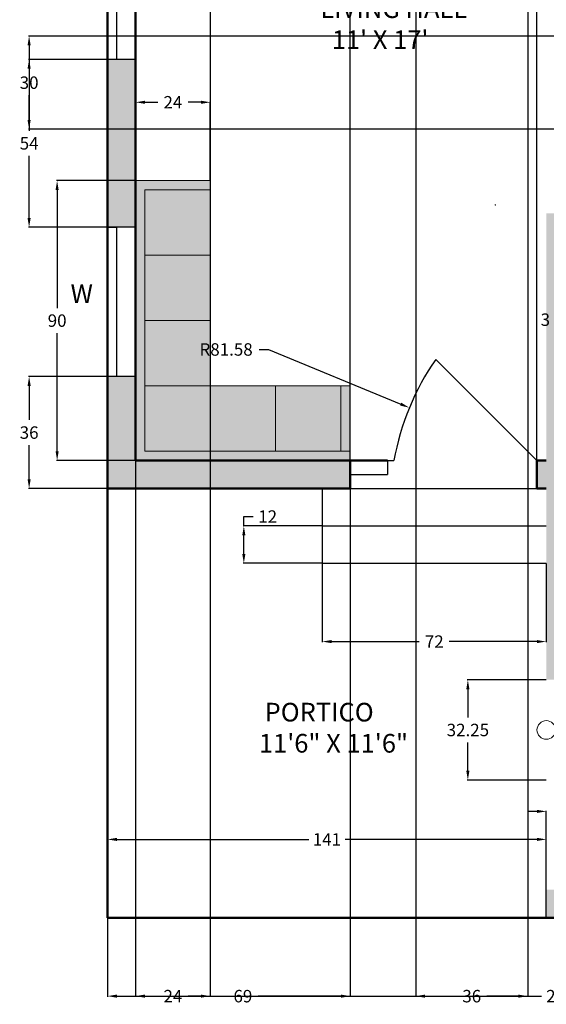
# Model space of a CAD drawing. Units: inches. Extents: x 30 to 385, y 81 to 626.
# Tile 1 of 4: x 30 to 199, y 81 to 398. Entities that reach past the tile are written whole.
import ezdxf

# ---------------------------------------------------------------- set-up
doc = ezdxf.new("R2010")
doc.units = ezdxf.units.IN
doc.header["$MEASUREMENT"] = 0
for name, color, linetype, lineweight in [('A-ANNO-DIMS', 2, 'Continuous', 18), ('A-ANNO-REF', 8, 'Continuous', 13), ('A-ANNO-SYMB', 7, 'Continuous', 18), ('A-ANNO-TEXT', 7, 'Continuous', 18), ('A-AREA-IDEN', 7, 'Continuous', 25), ('A-DOOR', 3, 'Continuous', 25), ('A-FLOR-STRS', 7, 'Continuous', 25), ('A-FURN', 8, 'Continuous', 18), ('A-GLAZ', 4, 'Continuous', 25), ('A-WALL', 7, 'Continuous', 50), ('A-WALL-PATT', 32, 'Continuous', 13)]:
    doc.layers.add(name, color=color, linetype=linetype, lineweight=lineweight)
doc.layers.add('A-FURN-PATT', color=254, linetype='Continuous', lineweight=13, true_color=0xfeeab9)
doc.styles.get("Standard").update_dxf_attribs({"font": 'arial.ttf'})
doc.dimstyles.get("Standard").update_dxf_attribs({"dimtxt": 4, "dimasz": 3, "dimexe": 0.18, "dimexo": 0.0625, "dimgap": 2, "dimtad": 0, "dimtih": 1, "dimtoh": 1, "dimdec": 0, "dimzin": 0, "dimdsep": 46, "dimlunit": 3, "dimtxsty": 'Standard', "dimcen": 0.09, "dimadec": 0, "dimazin": 0, "dimtfac": 1, "dimtdec": 0, "dimtofl": 0, "dimtmove": 0, "dimatfit": 3, "dimfxl": 1, "dimtolj": 1, "dimtzin": 0, "dimarcsym": 0})

# ---------------------------------------------------------------- blocks, each defined once
blk = doc.blocks.new('WIN-48')
for p, q in [((0, 0), (0, 9)), ((48, 0), (48, 9)), ((0, 6), (48, 6))]:
    blk.add_line(p, q)
blk = doc.blocks.new('*D16')
at = {"layer": 'A-ANNO-DIMS', "color": 0, "lineweight": -2, "transparency": 16777216}
for p, q in [((57.92, 109), (57.92, 83.68)), ((348.92, 109), (348.92, 83.68)), ((60.92, 83.86), (197.35, 83.86)), ((345.92, 83.86), (209.49, 83.86))]:
    blk.add_line(p, q, dxfattribs=at)
at = {"layer": 'A-ANNO-DIMS', "color": 0, "transparency": 16777216}
for points in [[(60.92, 84.36), (60.92, 83.36), (57.92, 83.86)], [(345.92, 84.36), (345.92, 83.36), (348.92, 83.86)]]:
    blk.add_solid(points, dxfattribs=at)
at = {"layer": 'Defpoints', "color": 0, "transparency": 16777216}
for p in [(57.92, 109.06), (348.92, 109.06), (348.92, 83.86)]:
    blk.add_point(p, dxfattribs=at)
at = {"layer": 'A-ANNO-DIMS', "color": 0, "transparency": 16777216, "insert": (203.42, 83.86), "char_height": 4, "attachment_point": 5}
blk.add_mtext('\\A1;291', dxfattribs=at)
blk = doc.blocks.new('*D18')
at = {"layer": 'A-ANNO-DIMS', "color": 0, "lineweight": -2, "transparency": 16777216}
for p, q in [((57.92, 109.13), (57.92, 134.44)), ((60.92, 134.26), (122.57, 134.26)), ((195.92, 134.26), (134.26, 134.26)), ((198.92, 109.13), (198.92, 134.44))]:
    blk.add_line(p, q, dxfattribs=at)
at = {"layer": 'A-ANNO-DIMS', "color": 0, "transparency": 16777216}
for points in [[(60.92, 134.76), (60.92, 133.76), (57.92, 134.26)], [(195.92, 134.76), (195.92, 133.76), (198.92, 134.26)]]:
    blk.add_solid(points, dxfattribs=at)
at = {"layer": 'Defpoints', "color": 0, "transparency": 16777216}
for p in [(198.92, 134.26), (57.92, 109.06), (198.92, 109.06)]:
    blk.add_point(p, dxfattribs=at)
at = {"layer": 'A-ANNO-DIMS', "color": 0, "transparency": 16777216, "insert": (128.42, 134.26), "char_height": 4, "attachment_point": 5}
blk.add_mtext('\\A1;141', dxfattribs=at)
blk = doc.blocks.new('*D23')
at = {"layer": 'A-ANNO-DIMS', "color": 0, "lineweight": -2, "transparency": 16777216}
for p, q in [((57.86, 283.06), (32.54, 283.06)), ((32.72, 280.06), (32.72, 269.11)), ((32.72, 250.06), (32.72, 261.02)), ((57.86, 247.06), (32.54, 247.06))]:
    blk.add_line(p, q, dxfattribs=at)
at = {"layer": 'A-ANNO-DIMS', "color": 0, "transparency": 16777216}
for points in [[(32.22, 280.06), (33.22, 280.06), (32.72, 283.06)], [(32.22, 250.06), (33.22, 250.06), (32.72, 247.06)]]:
    blk.add_solid(points, dxfattribs=at)
at = {"layer": 'Defpoints', "color": 0, "transparency": 16777216}
for p in [(32.72, 283.06), (57.92, 283.06), (57.92, 247.06)]:
    blk.add_point(p, dxfattribs=at)
at = {"layer": 'A-ANNO-DIMS', "color": 0, "transparency": 16777216, "insert": (32.72, 265.06), "char_height": 4, "attachment_point": 5}
blk.add_mtext('\\A1;36', dxfattribs=at)
blk = doc.blocks.new('*D24')
at = {"layer": 'A-ANNO-DIMS', "color": 0, "lineweight": -2, "transparency": 16777216}
for p, q in [((57.86, 385.06), (32.54, 385.06)), ((32.72, 382.06), (32.72, 362.1)), ((32.72, 334.06), (32.72, 354.03)), ((57.86, 331.06), (32.54, 331.06))]:
    blk.add_line(p, q, dxfattribs=at)
at = {"layer": 'A-ANNO-DIMS', "color": 0, "transparency": 16777216}
for points in [[(32.22, 382.06), (33.22, 382.06), (32.72, 385.06)], [(32.22, 334.06), (33.22, 334.06), (32.72, 331.06)]]:
    blk.add_solid(points, dxfattribs=at)
at = {"layer": 'Defpoints', "color": 0, "transparency": 16777216}
for p in [(32.72, 385.06), (57.92, 385.06), (57.92, 331.06)]:
    blk.add_point(p, dxfattribs=at)
at = {"layer": 'A-ANNO-DIMS', "color": 0, "transparency": 16777216, "insert": (32.72, 358.06), "char_height": 4, "attachment_point": 5}
blk.add_mtext('\\A1;54', dxfattribs=at)
blk = doc.blocks.new('*D28')
at = {"layer": 'A-ANNO-DIMS', "color": 0, "lineweight": -2, "transparency": 16777216}
for p, q in [((66.92, 469), (66.92, 83.68)), ((90.92, 469), (90.92, 83.68)), ((69.92, 83.86), (74.03, 83.86)), ((87.92, 83.86), (83.81, 83.86))]:
    blk.add_line(p, q, dxfattribs=at)
at = {"layer": 'A-ANNO-DIMS', "color": 0, "transparency": 16777216}
for points in [[(69.92, 84.36), (69.92, 83.36), (66.92, 83.86)], [(87.92, 84.36), (87.92, 83.36), (90.92, 83.86)]]:
    blk.add_solid(points, dxfattribs=at)
at = {"layer": 'Defpoints', "color": 0, "transparency": 16777216}
for p in [(66.92, 469.06), (90.92, 469.06), (90.92, 83.86)]:
    blk.add_point(p, dxfattribs=at)
at = {"layer": 'A-ANNO-DIMS', "color": 0, "transparency": 16777216, "insert": (78.92, 83.86), "char_height": 4, "attachment_point": 5}
blk.add_mtext('\\A1;24', dxfattribs=at)
blk = doc.blocks.new('*D32')
at = {"layer": 'A-ANNO-DIMS', "color": 0, "lineweight": -2, "transparency": 16777216}
for p, q in [((135.92, 247.13), (135.92, 623.44)), ((138.92, 623.26), (161.05, 623.26)), ((192.92, 623.26), (170.79, 623.26)), ((195.92, 247.13), (195.92, 623.44))]:
    blk.add_line(p, q, dxfattribs=at)
at = {"layer": 'A-ANNO-DIMS', "color": 0, "transparency": 16777216}
for points in [[(138.92, 623.76), (138.92, 622.76), (135.92, 623.26)], [(192.92, 623.76), (192.92, 622.76), (195.92, 623.26)]]:
    blk.add_solid(points, dxfattribs=at)
at = {"layer": 'Defpoints', "color": 0, "transparency": 16777216}
for p in [(195.92, 623.26), (135.92, 247.06), (195.92, 247.06)]:
    blk.add_point(p, dxfattribs=at)
at = {"layer": 'A-ANNO-DIMS', "color": 0, "transparency": 16777216, "insert": (165.92, 623.26), "char_height": 4, "attachment_point": 5}
blk.add_mtext('\\A1;60', dxfattribs=at)
blk = doc.blocks.new('*D33')
at = {"layer": 'A-ANNO-DIMS', "color": 0, "lineweight": -2, "transparency": 16777216}
for p, q in [((156.96, 460), (156.96, 83.68)), ((192.96, 460), (192.96, 83.68)), ((159.96, 83.86), (170.09, 83.86)), ((189.96, 83.86), (179.82, 83.86))]:
    blk.add_line(p, q, dxfattribs=at)
at = {"layer": 'A-ANNO-DIMS', "color": 0, "transparency": 16777216}
for points in [[(159.96, 84.36), (159.96, 83.36), (156.96, 83.86)], [(189.96, 84.36), (189.96, 83.36), (192.96, 83.86)]]:
    blk.add_solid(points, dxfattribs=at)
at = {"layer": 'Defpoints', "color": 0, "transparency": 16777216}
for p in [(156.96, 460.06), (192.96, 460.06), (192.96, 83.86)]:
    blk.add_point(p, dxfattribs=at)
at = {"layer": 'A-ANNO-DIMS', "color": 0, "transparency": 16777216, "insert": (174.96, 83.86), "char_height": 4, "attachment_point": 5}
blk.add_mtext('\\A1;36', dxfattribs=at)
blk = doc.blocks.new('*D37')
at = {"layer": 'A-ANNO-DIMS', "color": 0, "lineweight": -2, "transparency": 16777216}
for p, q in [((207.92, 326.5), (207.92, 301.18)), ((210.92, 326.5), (210.92, 301.18)), ((204.92, 301.36), (201.92, 301.36)), ((213.92, 301.36), (216.92, 301.36))]:
    blk.add_line(p, q, dxfattribs=at)
at = {"layer": 'A-ANNO-DIMS', "color": 0, "transparency": 16777216}
for points in [[(204.92, 301.86), (204.92, 300.86), (207.92, 301.36)], [(213.92, 301.86), (213.92, 300.86), (210.92, 301.36)]]:
    blk.add_solid(points, dxfattribs=at)
at = {"layer": 'Defpoints', "color": 0, "transparency": 16777216}
for p in [(207.92, 326.56), (210.92, 326.56), (207.92, 301.36)]:
    blk.add_point(p, dxfattribs=at)
at = {"layer": 'A-ANNO-DIMS', "color": 0, "transparency": 16777216, "insert": (198.61, 301.36), "char_height": 4, "attachment_point": 5}
blk.add_mtext('\\A1;3', dxfattribs=at)
blk = doc.blocks.new('*D40')
at = {"layer": 'A-ANNO-DIMS', "color": 0, "lineweight": -2, "transparency": 16777216}
for p, q in [((258.86, 392.56), (32.54, 392.56)), ((32.72, 389.56), (32.72, 381.61)), ((32.72, 365.56), (32.72, 373.52)), ((258.86, 362.56), (32.54, 362.56))]:
    blk.add_line(p, q, dxfattribs=at)
at = {"layer": 'A-ANNO-DIMS', "color": 0, "transparency": 16777216}
for points in [[(32.22, 389.56), (33.22, 389.56), (32.72, 392.56)], [(32.22, 365.56), (33.22, 365.56), (32.72, 362.56)]]:
    blk.add_solid(points, dxfattribs=at)
at = {"layer": 'Defpoints', "color": 0, "transparency": 16777216}
for p in [(32.72, 392.56), (258.92, 392.56), (258.92, 362.56)]:
    blk.add_point(p, dxfattribs=at)
at = {"layer": 'A-ANNO-DIMS', "color": 0, "transparency": 16777216, "insert": (32.72, 377.56), "char_height": 4, "attachment_point": 5}
blk.add_mtext('\\A1;30', dxfattribs=at)
blk = doc.blocks.new('*D45')
at = {"layer": 'A-ANNO-DIMS', "color": 0, "lineweight": -2, "transparency": 16777216}
for p, q in [((198.86, 185.56), (173.54, 185.56)), ((173.72, 182.56), (173.72, 173.48)), ((173.72, 156.31), (173.72, 165.4)), ((198.86, 153.31), (173.54, 153.31))]:
    blk.add_line(p, q, dxfattribs=at)
at = {"layer": 'A-ANNO-DIMS', "color": 0, "transparency": 16777216}
for points in [[(173.22, 182.56), (174.22, 182.56), (173.72, 185.56)], [(173.22, 156.31), (174.22, 156.31), (173.72, 153.31)]]:
    blk.add_solid(points, dxfattribs=at)
at = {"layer": 'Defpoints', "color": 0, "transparency": 16777216}
for p in [(173.72, 185.56), (198.92, 185.56), (198.92, 153.31)]:
    blk.add_point(p, dxfattribs=at)
at = {"layer": 'A-ANNO-DIMS', "color": 0, "transparency": 16777216, "insert": (173.72, 169.44), "char_height": 4, "attachment_point": 5}
blk.add_mtext('\\A1;32.25', dxfattribs=at)
blk = doc.blocks.new('*D46')
at = {"layer": 'A-ANNO-DIMS', "color": 0, "lineweight": -2, "transparency": 16777216}
for p, q in [((195.919029, 143.263849), (192.919029, 143.263849)), ((198.919029, 118.126349), (198.919029, 143.443849)), ((208.919029, 118.126349), (208.919029, 143.443849)), ((211.919029, 143.263849), (214.919029, 143.263849))]:
    blk.add_line(p, q, dxfattribs=at)
at = {"layer": 'A-ANNO-DIMS', "color": 0, "transparency": 16777216}
for points in [[(195.919029, 143.763849), (195.919029, 142.763849), (198.919029, 143.263849)], [(211.919029, 143.763849), (211.919029, 142.763849), (208.919029, 143.263849)]]:
    blk.add_solid(points, dxfattribs=at)
at = {"layer": 'Defpoints', "color": 0, "transparency": 16777216}
for p in [(208.919029, 143.263849), (198.919029, 118.063849), (208.919029, 118.063849)]:
    blk.add_point(p, dxfattribs=at)
at = {"layer": 'A-ANNO-DIMS', "color": 0, "transparency": 16777216, "insert": (203.919029, 143.263849), "char_height": 4, "attachment_point": 5}
blk.add_mtext('\\A1;10', dxfattribs=at)
blk = doc.blocks.new('*D47')
at = {"layer": 'A-ANNO-DIMS', "color": 0, "lineweight": -2, "transparency": 16777216}
for p, q in [((126.92, 223), (126.92, 197.68)), ((198.92, 223), (198.92, 197.68)), ((129.92, 197.86), (158.09, 197.86)), ((195.92, 197.86), (167.75, 197.86))]:
    blk.add_line(p, q, dxfattribs=at)
at = {"layer": 'A-ANNO-DIMS', "color": 0, "transparency": 16777216}
for points in [[(129.92, 198.36), (129.92, 197.36), (126.92, 197.86)], [(195.92, 198.36), (195.92, 197.36), (198.92, 197.86)]]:
    blk.add_solid(points, dxfattribs=at)
at = {"layer": 'Defpoints', "color": 0, "transparency": 16777216}
for p in [(126.92, 223.06), (198.92, 223.06), (126.92, 197.86)]:
    blk.add_point(p, dxfattribs=at)
at = {"layer": 'A-ANNO-DIMS', "color": 0, "transparency": 16777216, "insert": (162.92, 197.86), "char_height": 4, "attachment_point": 5}
blk.add_mtext('\\A1;72', dxfattribs=at)
blk = doc.blocks.new('*D48')
at = {"layer": 'A-ANNO-DIMS', "color": 0, "lineweight": -2, "transparency": 16777216}
for p, q in [((101.72, 235.06), (101.72, 238.06)), ((101.72, 238.06), (104.72, 238.06)), ((126.86, 235.06), (101.54, 235.06)), ((101.72, 226.06), (101.72, 232.06)), ((126.86, 223.06), (101.54, 223.06))]:
    blk.add_line(p, q, dxfattribs=at)
at = {"layer": 'A-ANNO-DIMS', "color": 0, "transparency": 16777216}
for points in [[(101.22, 232.06), (102.22, 232.06), (101.72, 235.06)], [(101.22, 226.06), (102.22, 226.06), (101.72, 223.06)]]:
    blk.add_solid(points, dxfattribs=at)
at = {"layer": 'Defpoints', "color": 0, "transparency": 16777216}
for p in [(101.72, 235.06), (126.92, 235.06), (126.92, 223.06)]:
    blk.add_point(p, dxfattribs=at)
at = {"layer": 'A-ANNO-DIMS', "color": 0, "transparency": 16777216, "insert": (109.38, 238.06), "char_height": 4, "attachment_point": 5}
blk.add_mtext('\\A1;12', dxfattribs=at)
blk = doc.blocks.new('*D49')
at = {"layer": 'A-ANNO-DIMS', "color": 0, "lineweight": -2, "transparency": 16777216}
for p, q in [((66.92, 346.13), (66.92, 371.44)), ((69.92, 371.26), (74.03, 371.26)), ((87.92, 371.26), (83.81, 371.26)), ((90.92, 346.13), (90.92, 371.44))]:
    blk.add_line(p, q, dxfattribs=at)
at = {"layer": 'A-ANNO-DIMS', "color": 0, "transparency": 16777216}
for points in [[(69.92, 371.76), (69.92, 370.76), (66.92, 371.26)], [(87.92, 371.76), (87.92, 370.76), (90.92, 371.26)]]:
    blk.add_solid(points, dxfattribs=at)
at = {"layer": 'Defpoints', "color": 0, "transparency": 16777216}
for p in [(90.92, 371.26), (66.92, 346.06), (90.92, 346.06)]:
    blk.add_point(p, dxfattribs=at)
at = {"layer": 'A-ANNO-DIMS', "color": 0, "transparency": 16777216, "insert": (78.92, 371.26), "char_height": 4, "attachment_point": 5}
blk.add_mtext('\\A1;24', dxfattribs=at)
blk = doc.blocks.new('*D50')
at = {"layer": 'A-ANNO-DIMS', "color": 0, "lineweight": -2, "transparency": 16777216}
for p, q in [((66.86, 346.06), (41.54, 346.06)), ((41.72, 343.06), (41.72, 305.11)), ((41.72, 259.06), (41.72, 297.02)), ((66.86, 256.06), (41.54, 256.06))]:
    blk.add_line(p, q, dxfattribs=at)
at = {"layer": 'A-ANNO-DIMS', "color": 0, "transparency": 16777216}
for points in [[(41.22, 343.06), (42.22, 343.06), (41.72, 346.06)], [(41.22, 259.06), (42.22, 259.06), (41.72, 256.06)]]:
    blk.add_solid(points, dxfattribs=at)
at = {"layer": 'Defpoints', "color": 0, "transparency": 16777216}
for p in [(41.72, 346.06), (66.92, 346.06), (66.92, 256.06)]:
    blk.add_point(p, dxfattribs=at)
at = {"layer": 'A-ANNO-DIMS', "color": 0, "transparency": 16777216, "insert": (41.72, 301.06), "char_height": 4, "attachment_point": 5}
blk.add_mtext('\\A1;90', dxfattribs=at)
blk = doc.blocks.new('*D51')
at = {"layer": 'A-ANNO-DIMS', "color": 0, "lineweight": -2, "transparency": 16777216}
for p, q in [((66.92, 256), (66.92, 83.68)), ((135.92, 256), (135.92, 83.68)), ((69.92, 83.86), (96.54, 83.86)), ((132.92, 83.86), (106.3, 83.86))]:
    blk.add_line(p, q, dxfattribs=at)
at = {"layer": 'A-ANNO-DIMS', "color": 0, "transparency": 16777216}
for points in [[(69.92, 84.36), (69.92, 83.36), (66.92, 83.86)], [(132.92, 84.36), (132.92, 83.36), (135.92, 83.86)]]:
    blk.add_solid(points, dxfattribs=at)
at = {"layer": 'Defpoints', "color": 0, "transparency": 16777216}
for p in [(66.92, 256.06), (135.92, 256.06), (135.92, 83.86)]:
    blk.add_point(p, dxfattribs=at)
at = {"layer": 'A-ANNO-DIMS', "color": 0, "transparency": 16777216, "insert": (101.42, 83.86), "char_height": 4, "attachment_point": 5}
blk.add_mtext('\\A1;69', dxfattribs=at)
blk = doc.blocks.new('*D54')
at = {"layer": 'A-ANNO-DIMS', "color": 0, "lineweight": -2, "transparency": 16777216}
for p, q in [((106.69, 291.78), (109.69, 291.78)), ((109.69, 291.78), (152.14, 274.2)), ((230.19, 241.83), (230.37, 241.83)), ((230.28, 241.74), (230.28, 241.92))]:
    blk.add_line(p, q, dxfattribs=at)
at = {"layer": 'A-ANNO-DIMS', "color": 0, "transparency": 16777216}
blk.add_solid([(152.33, 274.66), (151.95, 273.74), (154.91, 273.05)], dxfattribs=at)
at = {"layer": 'Defpoints', "color": 0, "transparency": 16777216}
for p in [(154.91, 273.05), (230.28, 241.83)]:
    blk.add_point(p, dxfattribs=at)
at = {"layer": 'A-ANNO-DIMS', "color": 0, "transparency": 16777216, "insert": (96.02, 291.78), "char_height": 4, "attachment_point": 5}
blk.add_mtext('\\A1;R81.58', dxfattribs=at)
blk = doc.blocks.new('*D55')
at = {"layer": 'A-ANNO-DIMS', "color": 0, "lineweight": -2, "transparency": 16777216}
for p, q in [((182.46, 338.32), (182.64, 338.32)), ((182.55, 338.23), (182.55, 338.41)), ((276.32, 299.47), (243.93, 312.89)), ((279.32, 299.47), (276.32, 299.47))]:
    blk.add_line(p, q, dxfattribs=at)
at = {"layer": 'A-ANNO-DIMS', "color": 0, "transparency": 16777216}
blk.add_solid([(244.12, 313.35), (243.73, 312.43), (241.15, 314.04)], dxfattribs=at)
at = {"layer": 'Defpoints', "color": 0, "transparency": 16777216}
for p in [(182.55, 338.32), (241.15, 314.04)]:
    blk.add_point(p, dxfattribs=at)
at = {"layer": 'A-ANNO-DIMS', "color": 0, "transparency": 16777216, "insert": (289.97, 299.47), "char_height": 4, "attachment_point": 5}
blk.add_mtext('\\A1;R63.44', dxfattribs=at)

msp = doc.modelspace()

# ---------------------------------------------------------------- hatches: boundary and pattern name
at = {"layer": 'A-FURN-PATT'}
h = msp.add_hatch(color=256, dxfattribs=at)
h.paths.add_polyline_path([(90.919, 343.0638), (69.919, 343.0638), (69.919, 322.0638), (90.919, 322.0638)], flags=17)
h.paths.add_polyline_path([(90.919, 322.0638), (69.919, 322.0638), (69.919, 301.0638), (90.919, 301.0638)], flags=17)
h.paths.add_polyline_path([(90.919, 301.0638), (69.919, 301.0638), (69.919, 280.0638), (90.919, 280.0638)], flags=17)
h.paths.add_polyline_path([(90.919, 280.0638), (69.919, 280.0638), (69.919, 259.0638), (90.919, 259.0638)], flags=17)
h.paths.add_polyline_path([(111.919, 280.0638), (90.919, 280.0638), (90.919, 259.0638), (111.919, 259.0638)], flags=17)
h.paths.add_polyline_path([(132.919, 280.0638), (111.919, 280.0638), (111.919, 259.0638), (132.919, 259.0638)], flags=17)
h.paths.add_polyline_path([(135.919, 280.0638), (132.919, 280.0638), (132.919, 259.0638), (135.919, 259.0638)])
h.paths.add_polyline_path([(135.919, 259.0638), (132.919, 259.0638), (69.919, 259.0638), (69.919, 280.0638), (69.919, 343.0638), (90.919, 343.0638), (90.919, 346.0638), (66.919, 346.0638), (66.919, 256.0638), (135.919, 256.0638)])
at = {"layer": 'A-WALL-PATT'}
h = msp.add_hatch(color=256, dxfattribs=at)
h.paths.add_polyline_path([(66.919, 385.0638), (57.919, 385.0638), (57.919, 331.0638), (60.919, 331.0638), (66.919, 331.0638)])
h.paths.add_polyline_path([(306.919, 469.0638), (249.919, 469.0638), (249.919, 460.0638), (258.919, 460.0638), (258.919, 392.5638), (267.919, 392.5638), (267.919, 395.5638), (339.919, 395.5638), (339.919, 377.5638), (348.919, 377.5638), (348.919, 418.0638), (339.919, 418.0638), (339.919, 400.0638), (267.919, 400.0638), (267.919, 460.0638), (306.919, 460.0638)])
h.paths.add_polyline_path([(339.919, 194.5638), (207.919, 194.5638), (207.919, 326.5638), (210.919, 326.5638), (210.919, 335.5638), (198.919, 335.5638), (198.919, 256.0638), (195.919, 256.0638), (195.919, 247.0638), (198.919, 247.0638), (198.919, 194.5638), (198.919, 185.5638), (339.919, 185.5638)])
h = msp.add_hatch(color=256, dxfattribs=at)
h.paths.add_polyline_path([(66.919, 283.0638), (57.919, 283.0638), (57.919, 247.0638), (66.919, 247.0638), (135.919, 247.0638), (135.919, 256.0638), (66.919, 256.0638)])
h.paths.add_polyline_path([(348.919, 275.5638), (339.919, 275.5638), (339.919, 118.0638), (198.919, 118.0638), (198.919, 109.0638), (348.919, 109.0638)])

# ---------------------------------------------------------------- linework, layer by layer
at = {"layer": 'A-ANNO-REF'}
for p in [(66.919, 392.0638), (66.919, 392.0638), (66.919, 324.0638), (66.919, 324.0638)]:
    msp.add_point(p, dxfattribs=at)
at = {"layer": 'A-ANNO-SYMB'}
msp.add_circle((198.919, 169.4388), 3, dxfattribs=at)
at = {"layer": 'A-DOOR'}
for p, q in [((195.919, 256.0638), (163.4136, 288.5693)), ((147.919, 256.0638), (147.919, 251.5638)), ((147.919, 256.0638), (149.9494, 256.0638)), ((135.919, 251.5638), (147.919, 251.5638)), ((135.919, 247.0638), (195.919, 247.0638))]:
    msp.add_line(p, q, dxfattribs=at)
msp.add_arc((230.2759, 241.8327), 81.5774, 145.046596, 169.953404, dxfattribs=at)
at = {"layer": 'A-FLOR-STRS'}
for p, q in [((126.919, 247.0638), (126.919, 223.0638)), ((126.919, 235.0638), (198.919, 235.0638)), ((126.919, 223.0638), (198.919, 223.0638))]:
    msp.add_line(p, q, dxfattribs=at)
at = {"layer": 'A-FURN'}
for p, q in [((90.919, 346.0638), (66.919, 346.0638)), ((90.919, 259.0638), (90.919, 346.0638)), ((69.919, 259.0638), (69.919, 343.0638)), ((90.919, 343.0638), (69.919, 343.0638)), ((90.919, 322.0638), (69.919, 322.0638)), ((90.919, 301.0638), (69.919, 301.0638)), ((135.919, 280.0638), (69.919, 280.0638)), ((111.919, 259.0638), (111.919, 280.0638)), ((132.919, 259.0638), (132.919, 280.0638)), ((135.919, 256.0638), (135.919, 280.0638)), ((135.919, 259.0638), (69.919, 259.0638))]:
    msp.add_line(p, q, dxfattribs=at)
at = {"layer": 'A-GLAZ'}
msp.add_line((57.919, 331.0638), (60.919, 331.0638), dxfattribs=at)
at = {"layer": 'A-WALL'}
for p, q in [((57.919, 598.0638), (57.919, 109.0638)), ((66.919, 460.0638), (66.919, 256.0638)), ((147.919, 256.0638), (66.919, 256.0638)), ((135.919, 256.0638), (135.919, 247.0638)), ((198.919, 256.0638), (195.919, 256.0638)), ((195.919, 256.0638), (195.919, 247.0638)), ((66.919, 247.0638), (57.919, 247.0638)), ((135.919, 247.0638), (66.919, 247.0638)), ((198.919, 247.0638), (195.919, 247.0638)), ((57.919, 109.0638), (348.919, 109.0638))]:
    msp.add_line(p, q, dxfattribs=at)

# ---------------------------------------------------------------- block references
at = {"layer": 'A-GLAZ'}
for p, rotation in [((66.919, 385.0638), 90.00000000000003), ((66.919, 283.0638), 89.99999999999999)]:
    msp.add_blockref('WIN-48', p, dxfattribs=dict(at, rotation=rotation))

# ---------------------------------------------------------------- texts
at = {"layer": 'A-ANNO-TEXT', "insert": (46.0278, 312.7297), "char_height": 6, "attachment_point": 1}
msp.add_mtext_dynamic_manual_height_columns('W', width=76.086845, gutter_width=1, heights=[0], dxfattribs=at)
at = {"layer": 'A-AREA-IDEN', "char_height": 6, "attachment_point": 1}
for s, insert in [("LIVING HALL\\P  11' X 17'", (126.3177, 404.3646)), (' PORTICO\\P11\'6" X 11\'6"', (106.5685, 178.173))]:
    msp.add_mtext_dynamic_manual_height_columns(s, width=76.086845, gutter_width=1, heights=[0], dxfattribs=dict(at, insert=insert))

# ---------------------------------------------------------------- dimensions: what is measured, and where the dimension line sits
at = {"layer": 'A-ANNO-DIMS'}
for base, p1, p2, picture, middle in [((195.919, 623.2638), (135.919, 247.0638), (195.919, 247.0638), '*D32', (165.919, 623.2638)), ((90.919, 83.8638), (66.919, 469.0638), (90.919, 469.0638), '*D28', (78.919, 83.8638)), ((192.9551, 83.8638), (156.9551, 460.0638), (192.9551, 460.0638), '*D33', (174.9551, 83.8638)), ((90.919, 371.2638), (66.919, 346.0638), (90.919, 346.0638), '*D49', (78.919, 371.2638)), ((135.919, 83.8638), (66.919, 256.0638), (135.919, 256.0638), '*D51', (101.419, 83.8638)), ((208.919, 143.2638), (198.919, 118.0638), (208.919, 118.0638), '*D46', (203.919, 143.2638)), ((198.919, 134.2638), (57.919, 109.0638), (198.919, 109.0638), '*D18', (128.419, 134.2638)), ((348.919, 83.8638), (57.919, 109.0638), (348.919, 109.0638), '*D16', (203.419, 83.8638))]:
    dim = msp.add_linear_dim(base=base, p1=p1, p2=p2, dimstyle='Standard', override={"dimdec": 0, "dimlfac": 1, "dimrnd": 0, "dimzin": 0, "dimdsep": 46, "dimlunit": 2}, dxfattribs=at)
    dim.commit()
    dim.dimension.update_dxf_attribs({"geometry": picture, "text_midpoint": middle})
for base, p1, p2, angle, override, picture, middle in [((32.719, 392.5638), (258.919, 362.5638), (258.919, 392.5638), 90, {"dimdec": 0, "dimlfac": 1, "dimrnd": 0, "dimzin": 0, "dimdsep": 46, "dimlunit": 2}, '*D40', (32.719, 377.5638)), ((32.719, 385.0638), (57.919, 331.0638), (57.919, 385.0638), 90, {"dimdec": 0, "dimlfac": 1, "dimrnd": 0, "dimzin": 0, "dimdsep": 46, "dimlunit": 2}, '*D24', (32.719, 358.0638)), ((41.719, 346.0638), (66.919, 256.0638), (66.919, 346.0638), 90, {"dimdec": 0, "dimlfac": 1, "dimrnd": 0, "dimzin": 0, "dimdsep": 46, "dimlunit": 2}, '*D50', (41.719, 301.0638)), ((207.919, 301.3638), (210.919, 326.5638), (207.919, 326.5638), 180, {"dimdec": 0, "dimlfac": 1, "dimrnd": 0, "dimzin": 0, "dimdsep": 46, "dimlunit": 2}, '*D37', (198.6093, 301.3638)), ((32.719, 283.0638), (57.919, 247.0638), (57.919, 283.0638), 90, {"dimdec": 0, "dimlfac": 1, "dimrnd": 0, "dimzin": 0, "dimdsep": 46, "dimlunit": 2}, '*D23', (32.719, 265.0638)), ((101.719, 235.0638), (126.919, 223.0638), (126.919, 235.0638), 90, {"dimdec": 0, "dimlfac": 1, "dimrnd": 0, "dimzin": 0, "dimdsep": 46, "dimlunit": 2}, '*D48', (109.3752, 238.0638)), ((126.919, 197.8638), (198.919, 223.0638), (126.919, 223.0638), 180, {"dimdec": 0, "dimlfac": 1, "dimrnd": 0, "dimzin": 0, "dimdsep": 46, "dimlunit": 2}, '*D47', (162.919, 197.8638)), ((173.719, 185.5638), (198.919, 153.3138), (198.919, 185.5638), 90, {"dimdec": 2, "dimlfac": 1, "dimrnd": 0, "dimzin": 0, "dimdsep": 46, "dimlunit": 2}, '*D45', (173.719, 169.4388))]:
    dim = msp.add_linear_dim(base=base, p1=p1, p2=p2, angle=angle, dimstyle='Standard', override=override, dxfattribs=at)
    dim.commit()
    dim.dimension.update_dxf_attribs({"geometry": picture, "text_midpoint": middle})
for center, mpoint, picture, middle in [((182.5453, 338.3166), (241.1541, 314.0399), '*D55', (289.9743, 299.4739)), ((230.2759, 241.8327), (154.9082, 273.0509), '*D54', (96.0204, 291.7818))]:
    dim = msp.add_radius_dim(center=center, mpoint=mpoint, dimstyle='Standard', override={"dimdec": 2, "dimlfac": 1, "dimrnd": 0, "dimzin": 0, "dimdsep": 46, "dimlunit": 2}, dxfattribs=at)
    dim.commit()
    dim.dimension.update_dxf_attribs({"geometry": picture, "text_midpoint": middle, "dimtype": 164})

doc.saveas('drawing.dxf')
